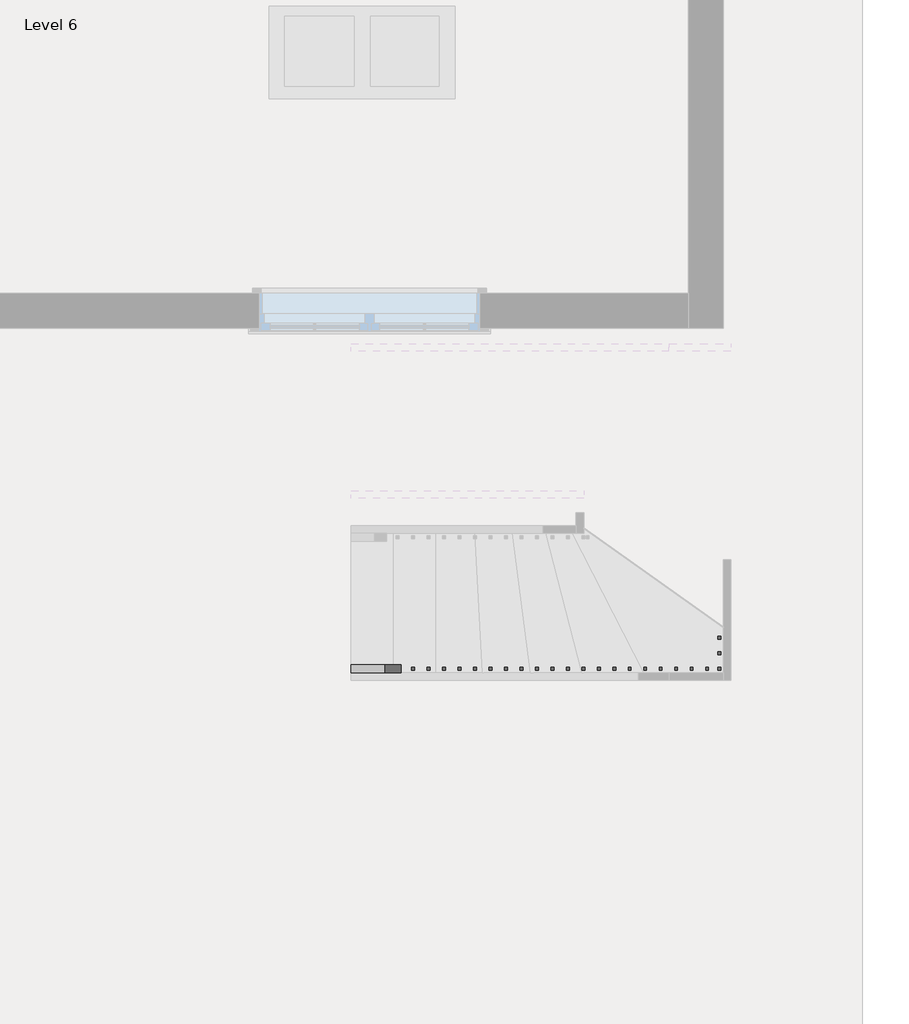
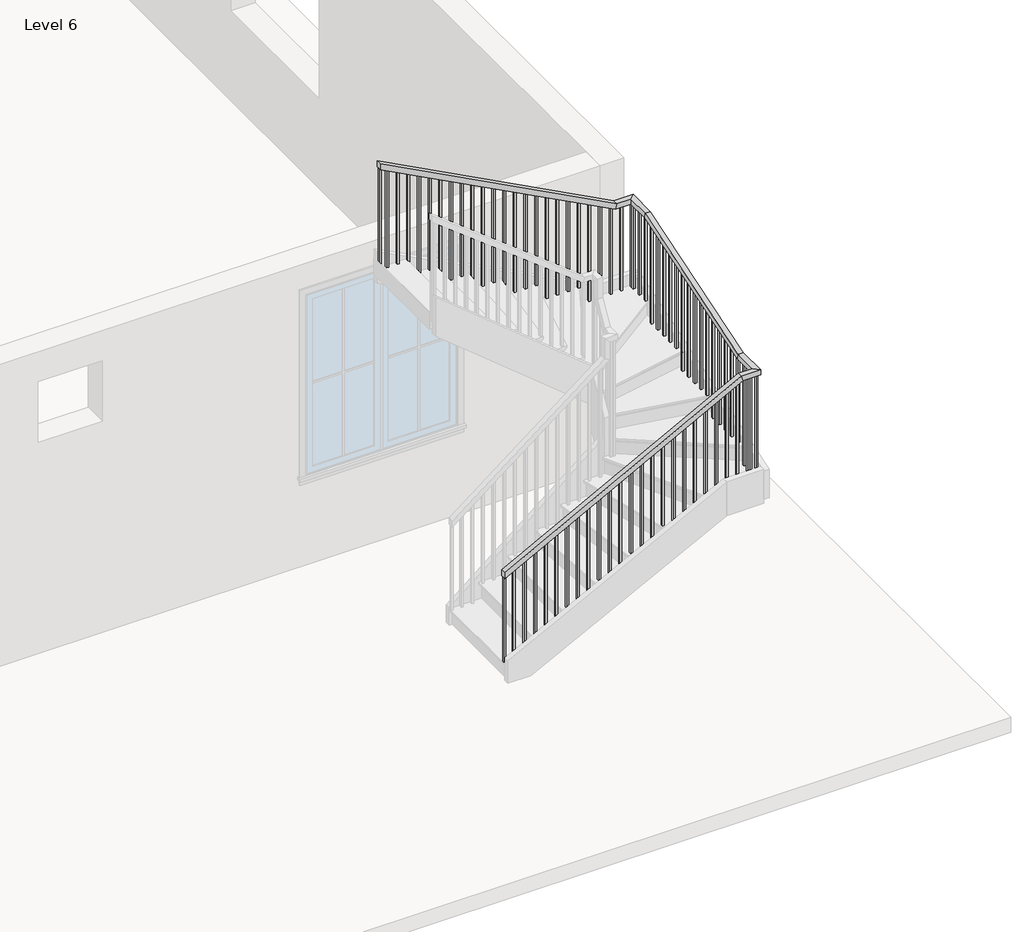
# One storey, part 2 of 3: 1 railing.
"""IFC4 building model written with IfcOpenShell, lengths in millimetres."""

from ifc_helpers import new_model, si_unit, frame, origin, place, context, project, spatial, polyline, outline, extrude, faceted_brep, element, save

model = new_model("IFC4")

# Units and contexts
model_context = context("Model", 3, world=origin())
ifc_project = project(units=[si_unit("LENGTHUNIT", "METRE", prefix="MILLI")], contexts=[model_context])

# Site, building, storey
site = spatial("IfcSite", under=ifc_project)
building = spatial("IfcBuilding", under=site)
storey = spatial("IfcBuildingStorey", under=building, Name="Level 6", Elevation=12801.6)

# Railing
placement = place(None, origin())
element("IfcRailing", 1, ObjectType="Handrail - Rectangular", at=placement, inside=storey, context=model_context, shape_type="SolidModel", body=[
    faceted_brep([(531.7538115, -7514.4090409, 13885.3333333), (531.7538115, -7514.4090409, 13827.8742652), (531.7538115, -7565.2090409, 13827.8742652), (531.7538115, -7565.2090409, 13885.3333333), (2789.4788736, -7514.4090409, 15078.6239201), (2802.0779381, -7514.4090409, 15027.8239201), (2802.0779381, -7565.2090409, 15027.8239201), (2789.4788736, -7565.2090409, 15078.6239201), (2923.0855034, -7269.9465826, 15027.8239201), (2923.0855034, -7277.8971587, 15078.6239201), (2923.0855034, -5744.320923, 15570.7094132), (2923.0855034, -5736.3703469, 15519.9094132), (2973.8855034, -7269.9465826, 15027.8239201), (2973.8855034, -5736.3703469, 15519.9094132), (2973.8855034, -7277.8971587, 15078.6239201), (2973.8855034, -5744.320923, 15570.7094132), (531.7538115, -5507.8090409, 16764.0), (531.7538115, -5457.0090409, 16764.0), (531.7538115, -5457.0090409, 16706.5409318), (531.7538115, -5507.8090409, 16706.5409318), (2776.879809, -5507.8090409, 15519.9094132), (2789.4788736, -5507.8090409, 15570.7094132), (2776.879809, -5457.0090409, 15519.9094132), (2789.4788736, -5457.0090409, 15570.7094132), (2923.0855034, -7514.4090409, 15078.6239201), (2923.0855034, -7514.4090409, 15027.8239201), (2973.8855034, -7565.2090409, 15027.8239201), (2973.8855034, -7565.2090409, 15078.6239201), (2923.0855034, -5507.8090409, 15570.7094132), (2923.0855034, -5507.8090409, 15519.9094132), (2973.8855034, -5457.0090409, 15519.9094132), (2973.8855034, -5457.0090409, 15570.7094132)], [[[0, 1, 2, 3]], [[1, 0, 4, 5]], [[2, 1, 5, 6]], [[3, 2, 6, 7]], [[0, 3, 7, 4]], [[8, 9, 10, 11]], [[12, 8, 11, 13]], [[14, 12, 13, 15]], [[9, 14, 15, 10]], [[16, 17, 18, 19]], [[20, 21, 16, 19]], [[22, 20, 19, 18]], [[23, 22, 18, 17]], [[21, 23, 17, 16]], [[5, 4, 24, 25]], [[6, 5, 25, 26]], [[7, 6, 26, 27]], [[4, 7, 27, 24]], [[25, 24, 9, 8]], [[26, 25, 8, 12]], [[27, 26, 12, 14]], [[24, 27, 14, 9]], [[11, 10, 28, 29]], [[13, 11, 29, 30]], [[15, 13, 30, 31]], [[10, 15, 31, 28]], [[29, 28, 21, 20]], [[30, 29, 20, 22]], [[31, 30, 22, 23]], [[28, 31, 23, 21]]]),
    extrude(outline(polyline([(16659.2597858, 621.2105034), (16669.3284102, 602.1605034), (15680.2666667, 602.1605034), (15680.2666667, 621.2105034), (16659.2597858, 621.2105034)])), frame((0.0, -5491.9340409, 0.0), z_axis=(0.0, 1.0, 0.0), x_axis=(0.0, 0.0, 1.0)), (0.0, 0.0, 1.0), 19.05),
    extrude(outline(polyline([(16605.5604556, 722.8105034), (16615.62908, 703.7605034), (15680.2666667, 703.7605034), (15680.2666667, 722.8105034), (16605.5604556, 722.8105034)])), frame((0.0, -5491.9340409, 0.0), z_axis=(0.0, 1.0, 0.0), x_axis=(0.0, 0.0, 1.0)), (0.0, 0.0, 1.0), 19.05),
    extrude(outline(polyline([(16551.8611254, 824.4105034), (16561.9297498, 805.3605034), (15510.9333333, 805.3605034), (15510.9333333, 824.4105034), (16551.8611254, 824.4105034)])), frame((0.0, -5491.9340409, 0.0), z_axis=(0.0, 1.0, 0.0), x_axis=(0.0, 0.0, 1.0)), (0.0, 0.0, 1.0), 19.05),
    extrude(outline(polyline([(16498.1617952, 926.0105034), (16508.2304196, 906.9605034), (15510.9333333, 906.9605034), (15510.9333333, 926.0105034), (16498.1617952, 926.0105034)])), frame((0.0, -5491.9340409, 0.0), z_axis=(0.0, 1.0, 0.0), x_axis=(0.0, 0.0, 1.0)), (0.0, 0.0, 1.0), 19.05),
    extrude(outline(polyline([(16444.462465, 1027.6105034), (16454.5310894, 1008.5605034), (15510.9333333, 1008.5605034), (15510.9333333, 1027.6105034), (16444.462465, 1027.6105034)])), frame((0.0, -5491.9340409, 0.0), z_axis=(0.0, 1.0, 0.0), x_axis=(0.0, 0.0, 1.0)), (0.0, 0.0, 1.0), 19.05),
    extrude(outline(polyline([(16390.7631348, 1129.2105034), (16400.8317592, 1110.1605034), (15341.6, 1110.1605034), (15341.6, 1129.2105034), (16390.7631348, 1129.2105034)])), frame((0.0, -5491.9340409, 0.0), z_axis=(0.0, 1.0, 0.0), x_axis=(0.0, 0.0, 1.0)), (0.0, 0.0, 1.0), 19.05),
    extrude(outline(polyline([(16337.0638046, 1230.8105034), (16347.132429, 1211.7605034), (15341.6, 1211.7605034), (15341.6, 1230.8105034), (16337.0638046, 1230.8105034)])), frame((0.0, -5491.9340409, 0.0), z_axis=(0.0, 1.0, 0.0), x_axis=(0.0, 0.0, 1.0)), (0.0, 0.0, 1.0), 19.05),
    extrude(outline(polyline([(16283.3644744, 1332.4105034), (16293.4330988, 1313.3605034), (15341.6, 1313.3605034), (15341.6, 1332.4105034), (16283.3644744, 1332.4105034)])), frame((0.0, -5491.9340409, 0.0), z_axis=(0.0, 1.0, 0.0), x_axis=(0.0, 0.0, 1.0)), (0.0, 0.0, 1.0), 19.05),
    extrude(outline(polyline([(16229.6651442, 1434.0105034), (16239.7337686, 1414.9605034), (15172.2666667, 1414.9605034), (15172.2666667, 1434.0105034), (16229.6651442, 1434.0105034)])), frame((0.0, -5491.9340409, 0.0), z_axis=(0.0, 1.0, 0.0), x_axis=(0.0, 0.0, 1.0)), (0.0, 0.0, 1.0), 19.05),
    extrude(outline(polyline([(16175.965814, 1535.6105034), (16186.0344384, 1516.5605034), (15172.2666667, 1516.5605034), (15172.2666667, 1535.6105034), (16175.965814, 1535.6105034)])), frame((0.0, -5491.9340409, 0.0), z_axis=(0.0, 1.0, 0.0), x_axis=(0.0, 0.0, 1.0)), (0.0, 0.0, 1.0), 19.05),
    extrude(outline(polyline([(16122.2664838, 1637.2105034), (16132.3351082, 1618.1605034), (15172.2666667, 1618.1605034), (15172.2666667, 1637.2105034), (16122.2664838, 1637.2105034)])), frame((0.0, -5491.9340409, 0.0), z_axis=(0.0, 1.0, 0.0), x_axis=(0.0, 0.0, 1.0)), (0.0, 0.0, 1.0), 19.05),
    extrude(outline(polyline([(16068.5671536, 1738.8105034), (16078.635778, 1719.7605034), (15002.9333333, 1719.7605034), (15002.9333333, 1738.8105034), (16068.5671536, 1738.8105034)])), frame((0.0, -5491.9340409, 0.0), z_axis=(0.0, 1.0, 0.0), x_axis=(0.0, 0.0, 1.0)), (0.0, 0.0, 1.0), 19.05),
    extrude(outline(polyline([(16014.8678234, 1840.4105034), (16024.9364478, 1821.3605034), (15002.9333333, 1821.3605034), (15002.9333333, 1840.4105034), (16014.8678234, 1840.4105034)])), frame((0.0, -5491.9340409, 0.0), z_axis=(0.0, 1.0, 0.0), x_axis=(0.0, 0.0, 1.0)), (0.0, 0.0, 1.0), 19.05),
    extrude(outline(polyline([(15961.1684932, 1942.0105034), (15971.2371176, 1922.9605034), (15002.9333333, 1922.9605034), (15002.9333333, 1942.0105034), (15961.1684932, 1942.0105034)])), frame((0.0, -5491.9340409, 0.0), z_axis=(0.0, 1.0, 0.0), x_axis=(0.0, 0.0, 1.0)), (0.0, 0.0, 1.0), 19.05),
    extrude(outline(polyline([(15907.469163, 2043.6105034), (15917.5377874, 2024.5605034), (15002.9333333, 2024.5605034), (15002.9333333, 2043.6105034), (15907.469163, 2043.6105034)])), frame((0.0, -5491.9340409, 0.0), z_axis=(0.0, 1.0, 0.0), x_axis=(0.0, 0.0, 1.0)), (0.0, 0.0, 1.0), 19.05),
    extrude(outline(polyline([(15853.7698328, 2145.2105034), (15863.8384572, 2126.1605034), (14833.6, 2126.1605034), (14833.6, 2145.2105034), (15853.7698328, 2145.2105034)])), frame((0.0, -5491.9340409, 0.0), z_axis=(0.0, 1.0, 0.0), x_axis=(0.0, 0.0, 1.0)), (0.0, 0.0, 1.0), 19.05),
    extrude(outline(polyline([(15800.0705026, 2246.8105034), (15810.139127, 2227.7605034), (14833.6, 2227.7605034), (14833.6, 2246.8105034), (15800.0705026, 2246.8105034)])), frame((0.0, -5491.9340409, 0.0), z_axis=(0.0, 1.0, 0.0), x_axis=(0.0, 0.0, 1.0)), (0.0, 0.0, 1.0), 19.05),
    extrude(outline(polyline([(15746.3711724, 2348.4105034), (15756.4397968, 2329.3605034), (14833.6, 2329.3605034), (14833.6, 2348.4105034), (15746.3711724, 2348.4105034)])), frame((0.0, -5491.9340409, 0.0), z_axis=(0.0, 1.0, 0.0), x_axis=(0.0, 0.0, 1.0)), (0.0, 0.0, 1.0), 19.05),
    extrude(outline(polyline([(15692.6718422, 2450.0105034), (15702.7404666, 2430.9605034), (14833.6, 2430.9605034), (14833.6, 2450.0105034), (15692.6718422, 2450.0105034)])), frame((0.0, -5491.9340409, 0.0), z_axis=(0.0, 1.0, 0.0), x_axis=(0.0, 0.0, 1.0)), (0.0, 0.0, 1.0), 19.05),
    extrude(outline(polyline([(15638.972512, 2551.6105034), (15649.0411364, 2532.5605034), (14664.2666667, 2532.5605034), (14664.2666667, 2551.6105034), (15638.972512, 2551.6105034)])), frame((0.0, -5491.9340409, 0.0), z_axis=(0.0, 1.0, 0.0), x_axis=(0.0, 0.0, 1.0)), (0.0, 0.0, 1.0), 19.05),
    extrude(outline(polyline([(15585.2731818, 2653.2105034), (15595.3418062, 2634.1605034), (14664.2666667, 2634.1605034), (14664.2666667, 2653.2105034), (15585.2731818, 2653.2105034)])), frame((0.0, -5491.9340409, 0.0), z_axis=(0.0, 1.0, 0.0), x_axis=(0.0, 0.0, 1.0)), (0.0, 0.0, 1.0), 19.05),
    extrude(outline(polyline([(15531.5738516, 2754.8105034), (15541.642476, 2735.7605034), (14664.2666667, 2735.7605034), (14664.2666667, 2754.8105034), (15531.5738516, 2754.8105034)])), frame((0.0, -5491.9340409, 0.0), z_axis=(0.0, 1.0, 0.0), x_axis=(0.0, 0.0, 1.0)), (0.0, 0.0, 1.0), 19.05),
    extrude(outline(polyline([(2856.4105034, -5472.8840409), (2856.4105034, -5491.9340409), (2837.3605034, -5491.9340409), (2837.3605034, -5472.8840409), (2856.4105034, -5472.8840409)])), frame((0.0, 0.0, 14664.2666667), z_axis=(0.0, 0.0, 1.0), x_axis=(1.0, 0.0, 0.0)), (0.0, 0.0, 1.0), 855.6427466),
    extrude(outline(polyline([(2958.0105034, -5517.3340409), (2938.9605034, -5517.3340409), (2938.9605034, -5498.2840409), (2958.0105034, -5498.2840409), (2958.0105034, -5517.3340409)])), frame((0.0, 0.0, 14664.2666667), z_axis=(0.0, 0.0, 1.0), x_axis=(1.0, 0.0, 0.0)), (0.0, 0.0, 1.0), 855.6427466),
    extrude(outline(polyline([(2958.0105034, -5618.9340409), (2938.9605034, -5618.9340409), (2938.9605034, -5599.8840409), (2958.0105034, -5599.8840409), (2958.0105034, -5618.9340409)])), frame((0.0, 0.0, 14664.2666667), z_axis=(0.0, 0.0, 1.0), x_axis=(1.0, 0.0, 0.0)), (0.0, 0.0, 1.0), 855.6427466),
    extrude(outline(polyline([(2958.0105034, -5720.5340409), (2938.9605034, -5720.5340409), (2938.9605034, -5701.4840409), (2958.0105034, -5701.4840409), (2958.0105034, -5720.5340409)])), frame((0.0, 0.0, 14664.2666667), z_axis=(0.0, 0.0, 1.0), x_axis=(1.0, 0.0, 0.0)), (0.0, 0.0, 1.0), 855.6427466),
    extrude(outline(polyline([(-5822.1340409, 15492.3900316), (-5803.0840409, 15498.5026907), (-5803.0840409, 14494.9333333), (-5822.1340409, 14494.9333333), (-5822.1340409, 15492.3900316)])), frame((2938.9605034, 0.0, 0.0), z_axis=(1.0, 0.0, 0.0), x_axis=(0.0, 1.0, 0.0)), (0.0, 0.0, 1.0), 19.05),
    extrude(outline(polyline([(-5923.7340409, 15459.7891834), (-5904.6840409, 15465.9018425), (-5904.6840409, 14494.9333333), (-5923.7340409, 14494.9333333), (-5923.7340409, 15459.7891834)])), frame((2938.9605034, 0.0, 0.0), z_axis=(1.0, 0.0, 0.0), x_axis=(0.0, 1.0, 0.0)), (0.0, 0.0, 1.0), 19.05),
    extrude(outline(polyline([(-6025.3340409, 15427.1883352), (-6006.2840409, 15433.3009942), (-6006.2840409, 14494.9333333), (-6025.3340409, 14494.9333333), (-6025.3340409, 15427.1883352)])), frame((2938.9605034, 0.0, 0.0), z_axis=(1.0, 0.0, 0.0), x_axis=(0.0, 1.0, 0.0)), (0.0, 0.0, 1.0), 19.05),
    extrude(outline(polyline([(-6126.9340409, 15394.587487), (-6107.8840409, 15400.700146), (-6107.8840409, 14494.9333333), (-6126.9340409, 14494.9333333), (-6126.9340409, 15394.587487)])), frame((2938.9605034, 0.0, 0.0), z_axis=(1.0, 0.0, 0.0), x_axis=(0.0, 1.0, 0.0)), (0.0, 0.0, 1.0), 19.05),
    extrude(outline(polyline([(-6228.5340409, 15361.9866387), (-6209.4840409, 15368.0992978), (-6209.4840409, 14494.9333333), (-6228.5340409, 14494.9333333), (-6228.5340409, 15361.9866387)])), frame((2938.9605034, 0.0, 0.0), z_axis=(1.0, 0.0, 0.0), x_axis=(0.0, 1.0, 0.0)), (0.0, 0.0, 1.0), 19.05),
    extrude(outline(polyline([(-6330.1340409, 15329.3857905), (-6311.0840409, 15335.4984495), (-6311.0840409, 14325.6), (-6330.1340409, 14325.6), (-6330.1340409, 15329.3857905)])), frame((2938.9605034, 0.0, 0.0), z_axis=(1.0, 0.0, 0.0), x_axis=(0.0, 1.0, 0.0)), (0.0, 0.0, 1.0), 19.05),
    extrude(outline(polyline([(-6431.7340409, 15296.7849423), (-6412.6840409, 15302.8976013), (-6412.6840409, 14325.6), (-6431.7340409, 14325.6), (-6431.7340409, 15296.7849423)])), frame((2938.9605034, 0.0, 0.0), z_axis=(1.0, 0.0, 0.0), x_axis=(0.0, 1.0, 0.0)), (0.0, 0.0, 1.0), 19.05),
    extrude(outline(polyline([(-6533.3340409, 15264.184094), (-6514.2840409, 15270.2967531), (-6514.2840409, 14325.6), (-6533.3340409, 14325.6), (-6533.3340409, 15264.184094)])), frame((2938.9605034, 0.0, 0.0), z_axis=(1.0, 0.0, 0.0), x_axis=(0.0, 1.0, 0.0)), (0.0, 0.0, 1.0), 19.05),
    extrude(outline(polyline([(-6634.9340409, 15231.5832458), (-6615.8840409, 15237.6959049), (-6615.8840409, 14325.6), (-6634.9340409, 14325.6), (-6634.9340409, 15231.5832458)])), frame((2938.9605034, 0.0, 0.0), z_axis=(1.0, 0.0, 0.0), x_axis=(0.0, 1.0, 0.0)), (0.0, 0.0, 1.0), 19.05),
    extrude(outline(polyline([(-6736.5340409, 15198.9823976), (-6717.4840409, 15205.0950566), (-6717.4840409, 14325.6), (-6736.5340409, 14325.6), (-6736.5340409, 15198.9823976)])), frame((2938.9605034, 0.0, 0.0), z_axis=(1.0, 0.0, 0.0), x_axis=(0.0, 1.0, 0.0)), (0.0, 0.0, 1.0), 19.05),
    extrude(outline(polyline([(-6838.1340409, 15166.3815494), (-6819.0840409, 15172.4942084), (-6819.0840409, 14156.2666667), (-6838.1340409, 14156.2666667), (-6838.1340409, 15166.3815494)])), frame((2938.9605034, 0.0, 0.0), z_axis=(1.0, 0.0, 0.0), x_axis=(0.0, 1.0, 0.0)), (0.0, 0.0, 1.0), 19.05),
    extrude(outline(polyline([(-6939.7340409, 15133.7807011), (-6920.6840409, 15139.8933602), (-6920.6840409, 14156.2666667), (-6939.7340409, 14156.2666667), (-6939.7340409, 15133.7807011)])), frame((2938.9605034, 0.0, 0.0), z_axis=(1.0, 0.0, 0.0), x_axis=(0.0, 1.0, 0.0)), (0.0, 0.0, 1.0), 19.05),
    extrude(outline(polyline([(-7041.3340409, 15101.1798529), (-7022.2840409, 15107.292512), (-7022.2840409, 14156.2666667), (-7041.3340409, 14156.2666667), (-7041.3340409, 15101.1798529)])), frame((2938.9605034, 0.0, 0.0), z_axis=(1.0, 0.0, 0.0), x_axis=(0.0, 1.0, 0.0)), (0.0, 0.0, 1.0), 19.05),
    extrude(outline(polyline([(-7142.9340409, 15068.5790047), (-7123.8840409, 15074.6916637), (-7123.8840409, 14156.2666667), (-7142.9340409, 14156.2666667), (-7142.9340409, 15068.5790047)])), frame((2938.9605034, 0.0, 0.0), z_axis=(1.0, 0.0, 0.0), x_axis=(0.0, 1.0, 0.0)), (0.0, 0.0, 1.0), 19.05),
    extrude(outline(polyline([(-7244.5340409, 15035.9781565), (-7225.4840409, 15042.0908155), (-7225.4840409, 14156.2666667), (-7244.5340409, 14156.2666667), (-7244.5340409, 15035.9781565)])), frame((2938.9605034, 0.0, 0.0), z_axis=(1.0, 0.0, 0.0), x_axis=(0.0, 1.0, 0.0)), (0.0, 0.0, 1.0), 19.05),
    extrude(outline(polyline([(2958.0105034, -7346.1340409), (2938.9605034, -7346.1340409), (2938.9605034, -7327.0840409), (2958.0105034, -7327.0840409), (2958.0105034, -7346.1340409)])), frame((0.0, 0.0, 13986.9333333), z_axis=(0.0, 0.0, 1.0), x_axis=(1.0, 0.0, 0.0)), (0.0, 0.0, 1.0), 1040.8905868),
    extrude(outline(polyline([(2958.0105034, -7447.7340409), (2938.9605034, -7447.7340409), (2938.9605034, -7428.6840409), (2958.0105034, -7428.6840409), (2958.0105034, -7447.7340409)])), frame((0.0, 0.0, 13986.9333333), z_axis=(0.0, 0.0, 1.0), x_axis=(1.0, 0.0, 0.0)), (0.0, 0.0, 1.0), 1040.8905868),
    extrude(outline(polyline([(2859.0288115, -7549.3340409), (2859.0288115, -7530.2840409), (2878.0788115, -7530.2840409), (2878.0788115, -7549.3340409), (2859.0288115, -7549.3340409)])), frame((0.0, 0.0, 13986.9333333), z_axis=(0.0, 0.0, 1.0), x_axis=(1.0, 0.0, 0.0)), (0.0, 0.0, 1.0), 1040.8905868),
    extrude(outline(polyline([(15014.2938418, 2776.4788115), (15004.2252174, 2757.4288115), (13986.9333333, 2757.4288115), (13986.9333333, 2776.4788115), (15014.2938418, 2776.4788115)])), frame((0.0, -7549.3340409, 0.0), z_axis=(0.0, 1.0, 0.0), x_axis=(0.0, 0.0, 1.0)), (0.0, 0.0, 1.0), 19.05),
    extrude(outline(polyline([(14960.5945116, 2674.8788115), (14950.5258872, 2655.8288115), (13986.9333333, 2655.8288115), (13986.9333333, 2674.8788115), (14960.5945116, 2674.8788115)])), frame((0.0, -7549.3340409, 0.0), z_axis=(0.0, 1.0, 0.0), x_axis=(0.0, 0.0, 1.0)), (0.0, 0.0, 1.0), 19.05),
    extrude(outline(polyline([(14906.8951814, 2573.2788115), (14896.826557, 2554.2288115), (13986.9333333, 2554.2288115), (13986.9333333, 2573.2788115), (14906.8951814, 2573.2788115)])), frame((0.0, -7549.3340409, 0.0), z_axis=(0.0, 1.0, 0.0), x_axis=(0.0, 0.0, 1.0)), (0.0, 0.0, 1.0), 19.05),
    extrude(outline(polyline([(14853.1958512, 2471.6788115), (14843.1272268, 2452.6288115), (13986.9333333, 2452.6288115), (13986.9333333, 2471.6788115), (14853.1958512, 2471.6788115)])), frame((0.0, -7549.3340409, 0.0), z_axis=(0.0, 1.0, 0.0), x_axis=(0.0, 0.0, 1.0)), (0.0, 0.0, 1.0), 19.05),
    extrude(outline(polyline([(14799.496521, 2370.0788115), (14789.4278966, 2351.0288115), (13817.6, 2351.0288115), (13817.6, 2370.0788115), (14799.496521, 2370.0788115)])), frame((0.0, -7549.3340409, 0.0), z_axis=(0.0, 1.0, 0.0), x_axis=(0.0, 0.0, 1.0)), (0.0, 0.0, 1.0), 19.05),
    extrude(outline(polyline([(14745.7971908, 2268.4788115), (14735.7285664, 2249.4288115), (13817.6, 2249.4288115), (13817.6, 2268.4788115), (14745.7971908, 2268.4788115)])), frame((0.0, -7549.3340409, 0.0), z_axis=(0.0, 1.0, 0.0), x_axis=(0.0, 0.0, 1.0)), (0.0, 0.0, 1.0), 19.05),
    extrude(outline(polyline([(14692.0978606, 2166.8788115), (14682.0292362, 2147.8288115), (13817.6, 2147.8288115), (13817.6, 2166.8788115), (14692.0978606, 2166.8788115)])), frame((0.0, -7549.3340409, 0.0), z_axis=(0.0, 1.0, 0.0), x_axis=(0.0, 0.0, 1.0)), (0.0, 0.0, 1.0), 19.05),
    extrude(outline(polyline([(14638.3985304, 2065.2788115), (14628.329906, 2046.2288115), (13817.6, 2046.2288115), (13817.6, 2065.2788115), (14638.3985304, 2065.2788115)])), frame((0.0, -7549.3340409, 0.0), z_axis=(0.0, 1.0, 0.0), x_axis=(0.0, 0.0, 1.0)), (0.0, 0.0, 1.0), 19.05),
    extrude(outline(polyline([(14584.6992002, 1963.6788115), (14574.6305758, 1944.6288115), (13648.2666667, 1944.6288115), (13648.2666667, 1963.6788115), (14584.6992002, 1963.6788115)])), frame((0.0, -7549.3340409, 0.0), z_axis=(0.0, 1.0, 0.0), x_axis=(0.0, 0.0, 1.0)), (0.0, 0.0, 1.0), 19.05),
    extrude(outline(polyline([(14530.99987, 1862.0788115), (14520.9312456, 1843.0288115), (13648.2666667, 1843.0288115), (13648.2666667, 1862.0788115), (14530.99987, 1862.0788115)])), frame((0.0, -7549.3340409, 0.0), z_axis=(0.0, 1.0, 0.0), x_axis=(0.0, 0.0, 1.0)), (0.0, 0.0, 1.0), 19.05),
    extrude(outline(polyline([(14477.3005398, 1760.4788115), (14467.2319154, 1741.4288115), (13648.2666667, 1741.4288115), (13648.2666667, 1760.4788115), (14477.3005398, 1760.4788115)])), frame((0.0, -7549.3340409, 0.0), z_axis=(0.0, 1.0, 0.0), x_axis=(0.0, 0.0, 1.0)), (0.0, 0.0, 1.0), 19.05),
    extrude(outline(polyline([(14423.6012096, 1658.8788115), (14413.5325852, 1639.8288115), (13478.9333333, 1639.8288115), (13478.9333333, 1658.8788115), (14423.6012096, 1658.8788115)])), frame((0.0, -7549.3340409, 0.0), z_axis=(0.0, 1.0, 0.0), x_axis=(0.0, 0.0, 1.0)), (0.0, 0.0, 1.0), 19.05),
    extrude(outline(polyline([(14369.9018794, 1557.2788115), (14359.833255, 1538.2288115), (13478.9333333, 1538.2288115), (13478.9333333, 1557.2788115), (14369.9018794, 1557.2788115)])), frame((0.0, -7549.3340409, 0.0), z_axis=(0.0, 1.0, 0.0), x_axis=(0.0, 0.0, 1.0)), (0.0, 0.0, 1.0), 19.05),
    extrude(outline(polyline([(14316.2025492, 1455.6788115), (14306.1339248, 1436.6288115), (13478.9333333, 1436.6288115), (13478.9333333, 1455.6788115), (14316.2025492, 1455.6788115)])), frame((0.0, -7549.3340409, 0.0), z_axis=(0.0, 1.0, 0.0), x_axis=(0.0, 0.0, 1.0)), (0.0, 0.0, 1.0), 19.05),
    extrude(outline(polyline([(14262.503219, 1354.0788115), (14252.4345946, 1335.0288115), (13309.6, 1335.0288115), (13309.6, 1354.0788115), (14262.503219, 1354.0788115)])), frame((0.0, -7549.3340409, 0.0), z_axis=(0.0, 1.0, 0.0), x_axis=(0.0, 0.0, 1.0)), (0.0, 0.0, 1.0), 19.05),
    extrude(outline(polyline([(14208.8038888, 1252.4788115), (14198.7352644, 1233.4288115), (13309.6, 1233.4288115), (13309.6, 1252.4788115), (14208.8038888, 1252.4788115)])), frame((0.0, -7549.3340409, 0.0), z_axis=(0.0, 1.0, 0.0), x_axis=(0.0, 0.0, 1.0)), (0.0, 0.0, 1.0), 19.05),
    extrude(outline(polyline([(14155.1045586, 1150.8788115), (14145.0359342, 1131.8288115), (13309.6, 1131.8288115), (13309.6, 1150.8788115), (14155.1045586, 1150.8788115)])), frame((0.0, -7549.3340409, 0.0), z_axis=(0.0, 1.0, 0.0), x_axis=(0.0, 0.0, 1.0)), (0.0, 0.0, 1.0), 19.05),
    extrude(outline(polyline([(14101.4052284, 1049.2788115), (14091.336604, 1030.2288115), (13140.2666667, 1030.2288115), (13140.2666667, 1049.2788115), (14101.4052284, 1049.2788115)])), frame((0.0, -7549.3340409, 0.0), z_axis=(0.0, 1.0, 0.0), x_axis=(0.0, 0.0, 1.0)), (0.0, 0.0, 1.0), 19.05),
    extrude(outline(polyline([(14047.7058982, 947.6788115), (14037.6372738, 928.6288115), (13140.2666667, 928.6288115), (13140.2666667, 947.6788115), (14047.7058982, 947.6788115)])), frame((0.0, -7549.3340409, 0.0), z_axis=(0.0, 1.0, 0.0), x_axis=(0.0, 0.0, 1.0)), (0.0, 0.0, 1.0), 19.05),
    extrude(outline(polyline([(13994.006568, 846.0788115), (13983.9379436, 827.0288115), (13140.2666667, 827.0288115), (13140.2666667, 846.0788115), (13994.006568, 846.0788115)])), frame((0.0, -7549.3340409, 0.0), z_axis=(0.0, 1.0, 0.0), x_axis=(0.0, 0.0, 1.0)), (0.0, 0.0, 1.0), 19.05),
    extrude(outline(polyline([(13940.3072378, 744.4788115), (13930.2386134, 725.4288115), (12970.9333333, 725.4288115), (12970.9333333, 744.4788115), (13940.3072378, 744.4788115)])), frame((0.0, -7549.3340409, 0.0), z_axis=(0.0, 1.0, 0.0), x_axis=(0.0, 0.0, 1.0)), (0.0, 0.0, 1.0), 19.05),
    extrude(outline(polyline([(13886.6079076, 642.8788115), (13876.5392831, 623.8288115), (12970.9333333, 623.8288115), (12970.9333333, 642.8788115), (13886.6079076, 642.8788115)])), frame((0.0, -7549.3340409, 0.0), z_axis=(0.0, 1.0, 0.0), x_axis=(0.0, 0.0, 1.0)), (0.0, 0.0, 1.0), 19.05),
    extrude(outline(polyline([(2958.0105034, -5491.9340409), (2938.9605034, -5491.9340409), (2938.9605034, -5472.8840409), (2958.0105034, -5472.8840409), (2958.0105034, -5491.9340409)])), frame((0.0, 0.0, 14664.2666667), z_axis=(0.0, 0.0, 1.0), x_axis=(1.0, 0.0, 0.0)), (0.0, 0.0, 1.0), 855.6427466),
    extrude(outline(polyline([(2938.9605034, -7549.3340409), (2938.9605034, -7530.2840409), (2958.0105034, -7530.2840409), (2958.0105034, -7549.3340409), (2938.9605034, -7549.3340409)])), frame((0.0, 0.0, 13986.9333333), z_axis=(0.0, 0.0, 1.0), x_axis=(1.0, 0.0, 0.0)), (0.0, 0.0, 1.0), 1040.8905868),
    extrude(outline(polyline([(16696.4723074, 550.8038115), (16706.5409318, 531.7538115), (15680.2666667, 531.7538115), (15680.2666667, 550.8038115), (16696.4723074, 550.8038115)])), frame((0.0, -5491.9340409, 0.0), z_axis=(0.0, 1.0, 0.0), x_axis=(0.0, 0.0, 1.0)), (0.0, 0.0, 1.0), 19.05),
    extrude(outline(polyline([(13837.9428896, 550.8038115), (13827.8742652, 531.7538115), (12970.9333333, 531.7538115), (12970.9333333, 550.8038115), (13837.9428896, 550.8038115)])), frame((0.0, -7549.3340409, 0.0), z_axis=(0.0, 1.0, 0.0), x_axis=(0.0, 0.0, 1.0)), (0.0, 0.0, 1.0), 19.05),
])

save(model, "model.ifc")

# Revit data of these elements
# Type "Handrail - Rectangular"
#   Assembly Code = "C2010400"
#   built-in parameter 1008612 = 0.0416667 (stored number, unit not read)
#   built-in parameter 1008611 = 0.0416667 (stored number, unit not read)
#   built-in parameter 1008609 = 0.333333 (stored number, unit not read)
#   built-in parameter 1008604 = 0.166667 (stored number, unit not read)
#   built-in parameter 1008603 = 0.166667 (stored number, unit not read)
#   Railing Height = 3' - 0"
#   built-in parameter 1008630 = 2
#   built-in parameter 1008610 = 2
#   built-in parameter 1008618 = Baluster - Square : 3/4"
# Element 1 (IfcRailing, "Handrail - Rectangular")
#   Phase Created = New Construction
